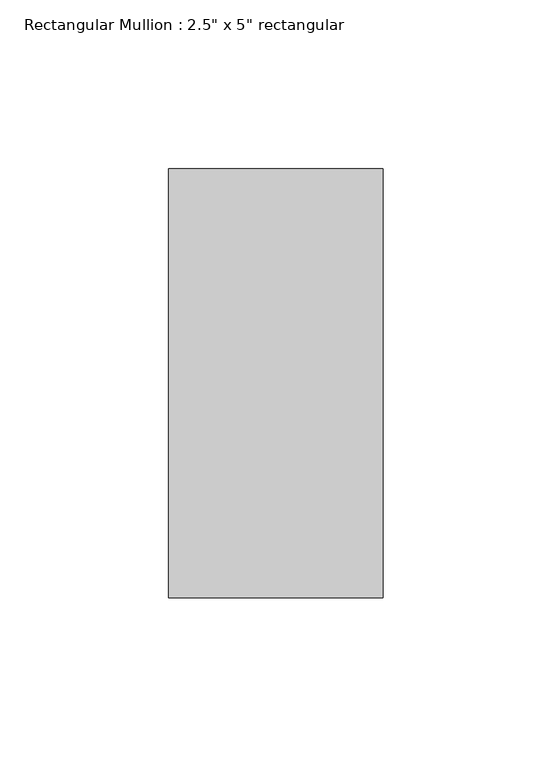
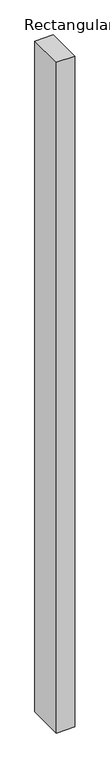
"""IFC4 building model written with IfcOpenShell, lengths in millimetres: member geometry."""

from ifc_helpers import new_model, si_unit, frame, origin, place, context, project, spatial, polyline, outline, extrude, source, transform, mapped, element, save


def member_5afaafd3(model_context):
    return source(origin(), model_context, "Body", "SweptSolid", [
        extrude(outline(polyline([(0.0, 63.5), (0.0, -63.5), (-63.5, -63.5), (-63.5, 63.5), (0.0, 63.5)])), frame((0.0, 0.0, -2428.9640157), z_axis=(0.0, 0.0, 1.0), x_axis=(1.0, 0.0, 0.0)), (0.0, 0.0, 1.0), 2428.9640157),
    ])


if __name__ == "__main__":
    model = new_model("IFC4")
    model_context = context("Model", 3, world=origin())
    ifc_project = project(units=[si_unit("LENGTHUNIT", "METRE", prefix="MILLI")], contexts=[model_context])
    site = spatial("IfcSite", under=ifc_project)
    building = spatial("IfcBuilding", under=site)
    placement = place(None, origin())
    member_shape = member_5afaafd3(model_context)
    element("IfcMember", 1, ObjectType="Rectangular Mullion : 2.5\" x 5\" rectangular", at=placement, inside=building, context=model_context, shape_type="MappedRepresentation", body=[
        mapped(member_shape, transform((0.0, 0.0, 0.0), x_axis=(1.0, 0.0, 0.0), y_axis=(0.0, 1.0, 0.0), z_axis=(0.0, 0.0, 1.0))),
    ])
    save(model, "model.ifc")

# Revit data of these elements
# Type "Rectangular Mullion : 2.5\" x 5\" rectangular"
#   built-in parameter 1007304 = 0.416667 (stored number, unit not read)
#   built-in parameter 1007301 = 0.104167 (stored number, unit not read)
#   built-in parameter 1007300 = 0.104167 (stored number, unit not read)
# Element 1 (IfcMember, "Rectangular Mullion : 2.5\" x 5\" rectangular")
#   Materials on its faces: "BLACK COLOUR"
# Materials
#   "BLACK COLOUR": class "Generic", colour RGB 120 120 120, transparency 0, Cost = 0
